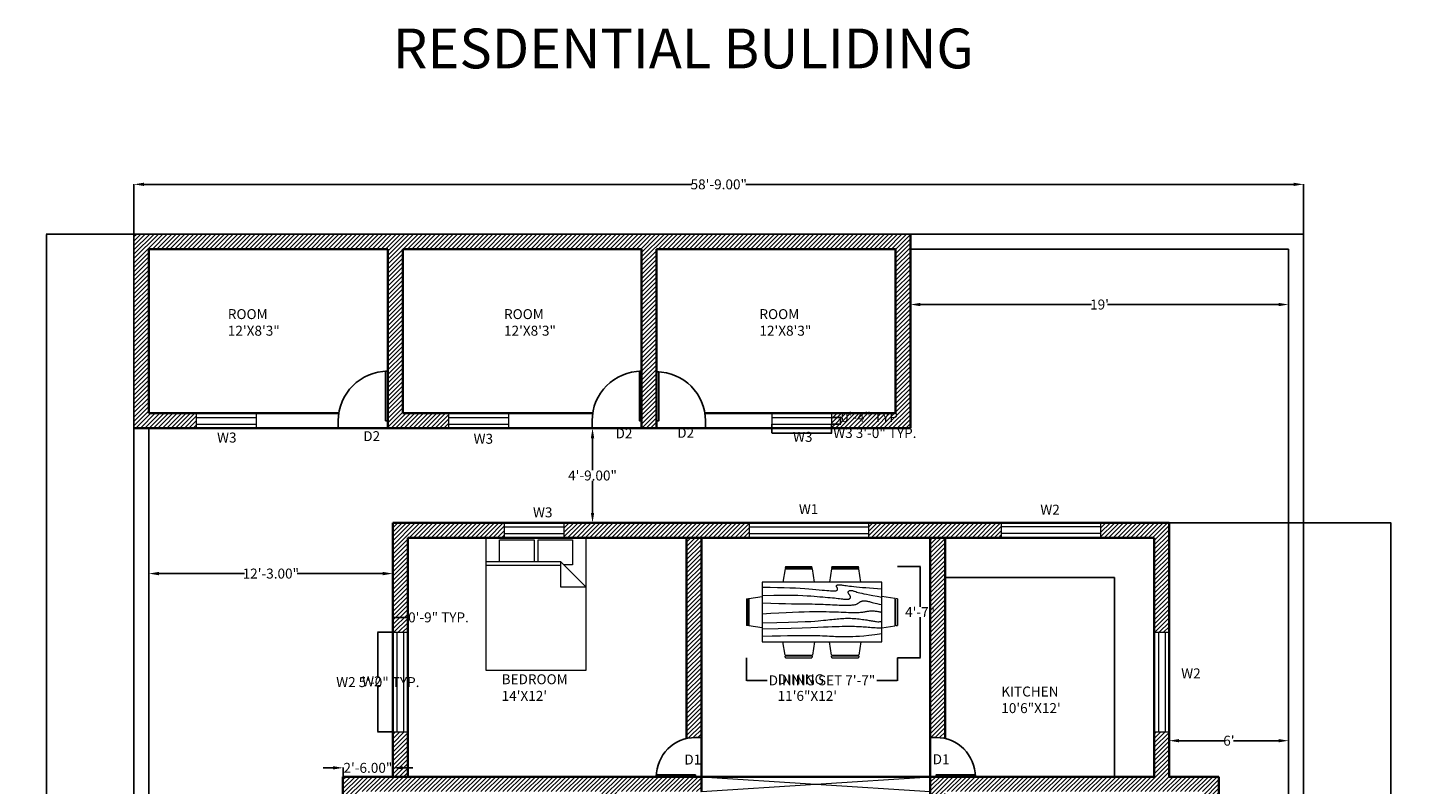
# Model space of a CAD drawing. Units: inches. Extents: x -57 to 1512, y -896 to 149.
# Tile 3 of 6: x -57 to 783, y -307 to 149. Entities that reach past the tile are written whole.
import ezdxf

# ---------------------------------------------------------------- set-up
doc = ezdxf.new("R2010")
doc.units = ezdxf.units.IN
doc.header["$MEASUREMENT"] = 0
doc.layers.get('Defpoints').update_dxf_attribs({"color": 9})
for name, color, linetype, lineweight in [('A-ANNO-DIMS', 2, 'Continuous', 18), ('A-ANNO-TEXT', 7, 'Continuous', 18), ('A-ANNO-TITL', 7, 'Continuous', 35), ('A-AREA-IDEN', 7, 'Continuous', 18), ('A-DOOR', 3, 'Continuous', 25), ('A-FLOR-CASE', 8, 'Continuous', 25), ('A-FURN', 8, 'Continuous', 18), ('A-GLAZ', 4, 'Continuous', 18), ('A-WALL', 7, 'Continuous', 35), ('A-WALL-OPEN', 7, 'Continuous', 18), ('A-WALL-PATT', 8, 'Continuous', 13), ('C-PROP', 7, 'Continuous', 25)]:
    doc.layers.add(name, color=color, linetype=linetype, lineweight=lineweight)
doc.styles.get("Standard").update_dxf_attribs({"font": 'arial.ttf'})
doc.dimstyles.get("Standard").update_dxf_attribs({"dimtxt": 6, "dimasz": 0.18, "dimexe": 0.18, "dimexo": 0.0625, "dimgap": 0.09, "dimtad": 0, "dimtih": 1, "dimtoh": 1, "dimzin": 0, "dimdsep": 46, "dimlunit": 3, "dimtxsty": 'Standard', "dimcen": 0.09, "dimadec": 0, "dimazin": 0, "dimtfac": 1, "dimtofl": 0, "dimtmove": 0, "dimatfit": 3, "dimfxl": 1, "dimtolj": 1, "dimtzin": 0, "dimarcsym": 0})

# ---------------------------------------------------------------- blocks, each defined once
blk = doc.blocks.new('*U2')
for p, q in [((0, 0), (0, -6)), ((40, 0), (40, -6))]:
    blk.add_line(p, q)
blk.add_lwpolyline([(0, 0), (0, 40), (1.75, 40), (1.75, 0)], close=True)
blk.add_arc((0, 0), 40, 0, 90)
blk = doc.blocks.new('Bed - Queen')
for p, q in [((0, -80.00003), (0, 0)), ((0, 0), (59.99999, 0)), ((59.99999, 0), (59.99999, -80.00003)), ((7.99999, -1.2), (28.79998, -1.2)), ((7.99999, -14.4), (7.99999, -1.2)), ((28.79998, -1.2), (28.79998, -14.4)), ((31.19999, -1.2), (51.99999, -1.2)), ((31.19999, -14.4), (31.19999, -1.2)), ((51.99999, -1.2), (51.99999, -16.4)), ((0, -14.4), (44.8, -14.4)), ((59.99999, -29.6), (44.8, -14.4)), ((44.8, -14.4), (44.8, -29.6)), ((51.99999, -16.4), (46.79936, -16.4)), ((44.8, -16.8), (0, -16.8)), ((44.8, -29.6), (59.99999, -29.6)), ((59.99999, -80.00003), (0, -80.00003))]:
    blk.add_line(p, q)
blk = doc.blocks.new('*D7')
at = {"layer": 'A-ANNO-DIMS', "color": 0, "lineweight": -2, "transparency": 16777216}
for p, q in [((283.51, -92.26), (283.88, -92.26)), ((283.7, -98.26), (283.7, -117.61)), ((283.7, -143.26), (283.7, -123.91)), ((283.51, -149.26), (283.88, -149.26))]:
    blk.add_line(p, q, dxfattribs=at)
at = {"layer": 'A-ANNO-DIMS', "color": 0, "transparency": 16777216}
for points in [[(282.7, -98.26), (284.7, -98.26), (283.7, -92.26)], [(282.7, -143.26), (284.7, -143.26), (283.7, -149.26)]]:
    blk.add_solid(points, dxfattribs=at)
at = {"layer": 'Defpoints', "color": 0, "transparency": 16777216}
for p in [(283.45, -92.26), (283.45, -149.26), (283.7, -149.26)]:
    blk.add_point(p, dxfattribs=at)
at = {"layer": 'A-ANNO-DIMS', "color": 0, "transparency": 16777216, "insert": (283.7, -120.76), "char_height": 6, "attachment_point": 5}
blk.add_mtext('\\A1;4\'-9.00"', dxfattribs=at)
blk = doc.blocks.new('*D8')
at = {"layer": 'A-ANNO-DIMS', "color": 0, "lineweight": -2, "transparency": 16777216}
for p, q in [((475.3, 15.68), (475.3, -17.9)), ((703.3, 15.68), (703.3, -17.9)), ((481.3, -17.72), (584.4, -17.72)), ((697.3, -17.72), (594.19, -17.72))]:
    blk.add_line(p, q, dxfattribs=at)
at = {"layer": 'A-ANNO-DIMS', "color": 0, "transparency": 16777216}
for points in [[(481.3, -16.72), (481.3, -18.72), (475.3, -17.72)], [(697.3, -16.72), (697.3, -18.72), (703.3, -17.72)]]:
    blk.add_solid(points, dxfattribs=at)
at = {"layer": 'Defpoints', "color": 0, "transparency": 16777216}
for p in [(475.3, 15.74), (703.3, 15.74), (703.3, -17.72)]:
    blk.add_point(p, dxfattribs=at)
at = {"layer": 'A-ANNO-DIMS', "color": 0, "transparency": 16777216, "insert": (589.3, -17.72), "char_height": 6, "attachment_point": 5}
blk.add_mtext("\\A1;19'", dxfattribs=at)
blk = doc.blocks.new('*D9')
at = {"layer": 'A-ANNO-DIMS', "color": 0, "lineweight": -2, "transparency": 16777216}
for p, q in [((661.3, -302.32), (661.3, -335.07)), ((703.3, -302.32), (703.3, -335.07)), ((667.3, -334.89), (668.41, -334.89)), ((697.3, -334.89), (696.18, -334.89))]:
    blk.add_line(p, q, dxfattribs=at)
at = {"layer": 'A-ANNO-DIMS', "color": 0, "transparency": 16777216}
for points in [[(667.3, -333.89), (667.3, -335.89), (661.3, -334.89)], [(697.3, -333.89), (697.3, -335.89), (703.3, -334.89)]]:
    blk.add_solid(points, dxfattribs=at)
at = {"layer": 'Defpoints', "color": 0, "transparency": 16777216}
for p in [(661.3, -302.26), (703.3, -302.26), (703.3, -334.89)]:
    blk.add_point(p, dxfattribs=at)
at = {"layer": 'A-ANNO-DIMS', "color": 0, "transparency": 16777216, "insert": (682.3, -334.89), "char_height": 6, "attachment_point": 5}
blk.add_mtext('\\A1;3\'-6.00"', dxfattribs=at)
blk = doc.blocks.new('*D18')
at = {"layer": 'A-ANNO-DIMS', "color": 0, "lineweight": -2, "transparency": 16777216}
for p, q in [((16.3, -149.32), (16.3, -180.04)), ((163.3, -149.32), (163.3, -180.04)), ((22.3, -179.86), (73.86, -179.86)), ((157.3, -179.86), (105.74, -179.86))]:
    blk.add_line(p, q, dxfattribs=at)
at = {"layer": 'A-ANNO-DIMS', "color": 0, "transparency": 16777216}
for points in [[(22.3, -178.86), (22.3, -180.86), (16.3, -179.86)], [(157.3, -178.86), (157.3, -180.86), (163.3, -179.86)]]:
    blk.add_solid(points, dxfattribs=at)
at = {"layer": 'Defpoints', "color": 0, "transparency": 16777216}
for p in [(16.3, -149.26), (163.3, -149.26), (16.3, -179.86)]:
    blk.add_point(p, dxfattribs=at)
at = {"layer": 'A-ANNO-DIMS', "color": 0, "transparency": 16777216, "insert": (89.8, -179.86), "char_height": 6, "attachment_point": 5}
blk.add_mtext('\\A1;12\'-3.00"', dxfattribs=at)
blk = doc.blocks.new('*D19')
at = {"layer": 'A-ANNO-DIMS', "color": 0, "lineweight": -2, "transparency": 16777216}
for p, q in [((16.3, -302.32), (16.3, -350.65)), ((133.3, -302.32), (133.3, -350.65)), ((22.3, -350.47), (60.91, -350.47)), ((127.3, -350.47), (88.69, -350.47))]:
    blk.add_line(p, q, dxfattribs=at)
at = {"layer": 'A-ANNO-DIMS', "color": 0, "transparency": 16777216}
for points in [[(22.3, -349.47), (22.3, -351.47), (16.3, -350.47)], [(127.3, -349.47), (127.3, -351.47), (133.3, -350.47)]]:
    blk.add_solid(points, dxfattribs=at)
at = {"layer": 'Defpoints', "color": 0, "transparency": 16777216}
for p in [(16.3, -302.26), (133.3, -302.26), (16.3, -350.47)]:
    blk.add_point(p, dxfattribs=at)
at = {"layer": 'A-ANNO-DIMS', "color": 0, "transparency": 16777216, "insert": (74.8, -350.47), "char_height": 6, "attachment_point": 5}
blk.add_mtext('\\A1;9\'-9.00"', dxfattribs=at)
blk = doc.blocks.new('*D20')
at = {"layer": 'A-ANNO-DIMS', "color": 0, "lineweight": -2, "transparency": 16777216}
for p, q in [((7.3, 24.8), (7.3, 54.88)), ((13.3, 54.7), (343.57, 54.7)), ((706.3, 54.7), (376.02, 54.7)), ((712.3, 24.8), (712.3, 54.88))]:
    blk.add_line(p, q, dxfattribs=at)
at = {"layer": 'A-ANNO-DIMS', "color": 0, "transparency": 16777216}
for points in [[(13.3, 55.7), (13.3, 53.7), (7.3, 54.7)], [(706.3, 55.7), (706.3, 53.7), (712.3, 54.7)]]:
    blk.add_solid(points, dxfattribs=at)
at = {"layer": 'Defpoints', "color": 0, "transparency": 16777216}
for p in [(7.3, 54.7), (7.3, 24.74), (712.3, 24.74)]:
    blk.add_point(p, dxfattribs=at)
at = {"layer": 'A-ANNO-DIMS', "color": 0, "transparency": 16777216, "insert": (359.8, 54.7), "char_height": 6, "attachment_point": 5}
blk.add_mtext('\\A1;58\'-9.00"', dxfattribs=at)
blk = doc.blocks.new('*D25')
at = {"layer": 'A-ANNO-DIMS', "color": 0, "lineweight": -2, "transparency": 16777216}
for p, q in [((631.3, -302.2), (631.3, -280.39)), ((637.3, -280.57), (664.43, -280.57)), ((697.3, -280.57), (670.16, -280.57)), ((703.3, -302.2), (703.3, -280.39))]:
    blk.add_line(p, q, dxfattribs=at)
at = {"layer": 'A-ANNO-DIMS', "color": 0, "transparency": 16777216}
for points in [[(637.3, -279.57), (637.3, -281.57), (631.3, -280.57)], [(697.3, -279.57), (697.3, -281.57), (703.3, -280.57)]]:
    blk.add_solid(points, dxfattribs=at)
at = {"layer": 'Defpoints', "color": 0, "transparency": 16777216}
for p in [(703.3, -280.57), (631.3, -302.26), (703.3, -302.26)]:
    blk.add_point(p, dxfattribs=at)
at = {"layer": 'A-ANNO-DIMS', "color": 0, "transparency": 16777216, "insert": (667.3, -280.57), "char_height": 6, "attachment_point": 5}
blk.add_mtext("\\A1;6'", dxfattribs=at)
blk = doc.blocks.new('*D26')
at = {"layer": 'A-ANNO-DIMS', "color": 0, "lineweight": -2, "transparency": 16777216}
for p, q in [((127.3, -296.93), (121.3, -296.93)), ((133.3, -302.2), (133.3, -296.75)), ((163.3, -302.2), (163.3, -296.75)), ((169.3, -296.93), (175.3, -296.93))]:
    blk.add_line(p, q, dxfattribs=at)
at = {"layer": 'A-ANNO-DIMS', "color": 0, "transparency": 16777216}
for points in [[(127.3, -295.93), (127.3, -297.93), (133.3, -296.93)], [(169.3, -295.93), (169.3, -297.93), (163.3, -296.93)]]:
    blk.add_solid(points, dxfattribs=at)
at = {"layer": 'Defpoints', "color": 0, "transparency": 16777216}
for p in [(163.3, -296.93), (133.3, -302.26), (163.3, -302.26)]:
    blk.add_point(p, dxfattribs=at)
at = {"layer": 'A-ANNO-DIMS', "color": 0, "transparency": 16777216, "insert": (148.3, -296.93), "char_height": 6, "attachment_point": 5}
blk.add_mtext('\\A1;2\'-6.00"', dxfattribs=at)
blk = doc.blocks.new('Dining Set - 36 x 72 in.')
for p, q in [((-22.2343, 26.00059), (-23.4847, 17.99762)), ((-22.2304, 26), (-5.7608, 26)), ((-22, 27.5), (-22.1562, 26.50042)), ((-5.8416, 26.5), (-22.1534, 26.5)), ((-22, 27.5), (-6, 27.5)), ((-5.8437, 26.49966), (-6, 27.5)), ((-4.5152, 17.99762), (-5.7655, 25.99926)), ((5.7657, 26.00059), (4.5153, 17.99762)), ((5.7696, 26), (22.2392, 26)), ((6, 27.5), (5.8438, 26.50042)), ((22.1584, 26.5), (5.8466, 26.5)), ((6, 27.5), (22, 27.5)), ((22.1563, 26.49966), (22, 27.5)), ((23.4848, 17.99762), (22.2345, 25.99926)), ((36, 18), (-36, 18)), ((-36, 18), (-36, -18)), ((36, -18), (36, 18)), ((-44.0006, 8.23428), (-35.9976, 9.48474)), ((44.0006, 8.23428), (35.9976, 9.48474)), ((-45.5, 8), (-44.5004, 8.15617)), ((-45.5, 8), (-45.5, -8)), ((-44.5, -8.15843), (-44.5, 8.15338)), ((-44, 8.23041), (-44, -8.23915)), ((44, 8.23041), (44, -8.23915)), ((44.5, -8.15843), (44.5, 8.15338)), ((45.5, 8), (44.5005, 8.15617)), ((45.5, 8), (45.5, -8)), ((-44.4997, -8.15631), (-45.5, -8)), ((-35.9976, -9.48476), (-43.9993, -8.2345)), ((35.9976, -9.48476), (43.9993, -8.2345)), ((44.4997, -8.15631), (45.5, -8)), ((-36, -18), (36, -18)), ((-22.2343, -26.0006), (-23.4847, -17.99762)), ((-4.5152, -17.99762), (-5.7655, -25.99928)), ((5.7657, -26.0006), (4.5153, -17.99762)), ((23.4848, -17.99762), (22.2345, -25.99928)), ((-22.2304, -26), (-5.7608, -26)), ((-22, -27.5), (-22.1562, -26.50044)), ((-5.8416, -26.5), (-22.1534, -26.5)), ((-22, -27.5), (-6, -27.5)), ((-5.8437, -26.49967), (-6, -27.5)), ((5.7696, -26), (22.2392, -26)), ((6, -27.5), (5.8438, -26.50044)), ((22.1584, -26.5), (5.8466, -26.5)), ((6, -27.5), (22, -27.5)), ((22.1563, -26.49967), (22, -27.5))]:
    blk.add_line(p, q)
for points in [[(-36, 15), (-31.1772, 14.97754), (-26.8079, 14.91406), (-22.8538, 14.81543), (-19.276, 14.6875), (-16.0362, 14.53613), (-13.0957, 14.36718), (-10.4159, 14.18652), (-7.9583, 14), (-5.6904, 13.81315), (-3.6035, 13.63021), (-1.6954, 13.45508), (0.0365, 13.29166), (1.5945, 13.14388), (2.9811, 13.01562), (4.1988, 12.9108), (5.25, 12.83333), (6.1393, 12.78613), (6.8802, 12.76823), (7.4883, 12.77767), (7.9792, 12.8125), (8.3685, 12.87077), (8.6719, 12.95052), (8.9049, 13.0498), (9.0833, 13.16666), (9.2205, 13.29899), (9.3216, 13.44401), (9.3895, 13.59879), (9.4271, 13.76041), (9.4373, 13.92594), (9.4232, 14.09245), (9.3875, 14.257), (9.3333, 14.41666), (9.2638, 14.56917), (9.1836, 14.71484), (9.0975, 14.85465), (9.0104, 14.98958), (8.9272, 15.1206), (8.8529, 15.2487), (8.7922, 15.37483), (8.75, 15.5), (8.7305, 15.62467), (8.7344, 15.74739), (8.7617, 15.86621), (8.8125, 15.97916), (8.8867, 16.08431), (8.9844, 16.17968), (9.1055, 16.26334), (9.25, 16.33333), (9.4189, 16.38802), (9.6172, 16.42708), (9.8506, 16.45052), (10.125, 16.45833), (10.4463, 16.45052), (10.8203, 16.42708), (11.2529, 16.38802), (11.75, 16.33333), (12.3184, 16.26318), (12.9694, 16.17838), (13.7151, 16.07991), (14.5677, 15.96875), (15.5395, 15.84586), (16.6426, 15.71224), (17.8893, 15.56884), (19.2917, 15.41666), (20.859, 15.25667), (22.5879, 15.08984), (24.4721, 14.91715), (26.5052, 14.73958), (28.6809, 14.5581), (30.9929, 14.3737), (33.4347, 14.18733), (36, 14)], [(-36, 10), (-28.9766, 10.14274), (-23.1725, 10.20442), (-18.4241, 10.19775), (-14.5677, 10.13541), (-11.4399, 10.03011), (-8.877, 9.89453), (-6.7154, 9.74137), (-4.7917, 9.58333), (-2.9698, 9.43082), (-1.2246, 9.28515), (0.4415, 9.14534), (2.026, 9.01041), (3.5266, 8.87939), (4.9408, 8.7513), (6.266, 8.62516), (7.5, 8.5), (8.6411, 8.37549), (9.6914, 8.2539), (10.6538, 8.13818), (11.5312, 8.03125), (12.3267, 7.93603), (13.043, 7.85547), (13.6831, 7.79248), (14.25, 7.75), (14.7471, 7.7303), (15.1797, 7.73307), (15.5537, 7.75732), (15.875, 7.80208), (16.1494, 7.86637), (16.3828, 7.94922), (16.5811, 8.04964), (16.75, 8.16666), (16.8944, 8.29915), (17.0143, 8.44531), (17.1089, 8.60319), (17.1771, 8.77083), (17.218, 8.94629), (17.2305, 9.1276), (17.2137, 9.31282), (17.1667, 9.5), (17.0895, 9.6875), (16.987, 9.875), (16.8649, 10.0625), (16.7292, 10.25), (16.5856, 10.4375), (16.4401, 10.625), (16.2985, 10.8125), (16.1667, 11), (16.05, 11.18733), (15.9518, 11.3737), (15.8752, 11.5581), (15.8229, 11.73958), (15.798, 11.91715), (15.8034, 12.08984), (15.842, 12.25667), (15.9167, 12.41666), (16.0295, 12.56836), (16.1784, 12.70833), (16.3605, 12.83268), (16.5729, 12.9375), (16.8127, 13.01888), (17.0768, 13.07291), (17.3625, 13.0957), (17.6667, 13.08333), (17.9894, 13.03312), (18.3418, 12.94726), (18.7382, 12.82918), (19.1927, 12.68229), (19.7195, 12.51001), (20.3327, 12.31575), (21.0465, 12.10294), (21.875, 11.875), (22.8357, 11.63354), (23.959, 11.37304), (25.2786, 11.08618), (26.8282, 10.76562), (28.6414, 10.40405), (30.752, 9.99414), (33.1936, 9.52856), (36, 9)], [(-36, 5.5), (-30.7157, 5.3348), (-26.069, 5.20963), (-21.9946, 5.11767), (-18.4271, 5.05208), (-15.3009, 5.00602), (-12.5508, 4.97265), (-10.1112, 4.94515), (-7.9167, 4.91666), (-5.909, 4.88167), (-4.0586, 4.83984), (-2.3429, 4.79215), (-0.7396, 4.73958), (0.7739, 4.6831), (2.22, 4.6237), (3.6213, 4.56233), (5, 4.5), (6.373, 4.43782), (7.7344, 4.3776), (9.0723, 4.32129), (10.375, 4.27083), (11.6309, 4.22819), (12.8281, 4.19531), (13.9551, 4.17415), (15, 4.16666), (15.954, 4.17448), (16.819, 4.19791), (17.6001, 4.23698), (18.3021, 4.29166), (18.9299, 4.36198), (19.4883, 4.44791), (19.9823, 4.54948), (20.4167, 4.66666), (20.7969, 4.79899), (21.1302, 4.94401), (21.4245, 5.09879), (21.6875, 5.26041), (21.9271, 5.42594), (22.1511, 5.59245), (22.3672, 5.757), (22.5834, 5.91666), (22.8065, 6.06868), (23.0404, 6.21093), (23.2879, 6.34147), (23.5521, 6.45833), (23.8358, 6.55957), (24.142, 6.64323), (24.4735, 6.70735), (24.8334, 6.75), (25.2235, 6.76969), (25.642, 6.76692), (26.0858, 6.74267), (26.5521, 6.69791), (27.0379, 6.63362), (27.5404, 6.55078), (28.0565, 6.45036), (28.5834, 6.33333), (29.1242, 6.19987), (29.7071, 6.04687), (30.3661, 5.87044), (31.1354, 5.66666), (32.0493, 5.43164), (33.142, 5.16146), (34.4475, 4.85221), (36, 4.5)], [(-36, -1), (-30.7915, -0.6591), (-26.0195, -0.38216), (-21.6519, -0.16284), (-17.6563, 0.00521), (-14.0005, 0.12833), (-10.6523, 0.21289), (-7.5796, 0.26522), (-4.75, 0.29166), (-2.134, 0.29793), (0.2878, 0.28711), (2.5317, 0.26163), (4.6146, 0.22396), (6.5529, 0.17651), (8.3633, 0.12174), (10.0623, 0.06209), (11.6667, 0), (13.1899, -0.06201), (14.6341, -0.1211), (15.9982, -0.17432), (17.2813, -0.21875), (18.4823, -0.25147), (19.6003, -0.26953), (20.6343, -0.27002), (21.5834, -0.25), (22.4481, -0.20768), (23.2357, -0.14584), (23.9549, -0.06836), (24.6146, 0.02083), (25.2235, 0.11784), (25.7904, 0.21875), (26.3241, 0.31966), (26.8334, 0.41666), (27.3265, 0.50618), (27.8099, 0.58593), (28.2894, 0.65397), (28.7709, 0.70833), (29.2601, 0.74707), (29.763, 0.76823), (30.2855, 0.76985), (30.8334, 0.75), (31.4088, 0.70784), (31.9994, 0.64713), (32.589, 0.57275), (33.1615, 0.48958), (33.7008, 0.4025), (34.1908, 0.3164), (34.6153, 0.23616), (34.9584, 0.16666), (35.2099, 0.11165), (35.3848, 0.07031), (35.504, 0.04069), (35.5886, 0.02083), (35.6594, 0.00879), (35.7377, 0.0026), (35.8442, 0.00032), (36, 0)], [(-36, -6.5), (-27.1843, -6.31267), (-20.084, -6.1263), (-14.469, -5.9419), (-10.1094, -5.76042), (-6.7752, -5.58285), (-4.2363, -5.41016), (-2.2629, -5.24333), (-0.625, -5.08334), (0.8708, -4.93099), (2.2715, -4.78646), (3.5872, -4.64974), (4.8281, -4.52084), (6.0046, -4.39974), (7.127, -4.28646), (8.2053, -4.18099), (9.25, -4.08334), (10.2705, -3.99382), (11.2734, -3.91407), (12.2647, -3.84603), (13.25, -3.79167), (14.2354, -3.75293), (15.2266, -3.73177), (16.2295, -3.73015), (17.25, -3.75), (18.2912, -3.79248), (19.3451, -3.85547), (20.4009, -3.93604), (21.4479, -4.03125), (22.4754, -4.13819), (23.4727, -4.25391), (24.4289, -4.37549), (25.3334, -4.5), (26.1785, -4.62492), (26.9694, -4.74935), (27.7145, -4.87281), (28.4219, -4.99479), (29.1, -5.11483), (29.7572, -5.23242), (30.4016, -5.34709), (31.0417, -5.45834), (31.6837, -5.56437), (32.3262, -5.65821), (32.9658, -5.73153), (33.599, -5.77604), (34.2224, -5.78345), (34.8327, -5.74545), (35.4264, -5.65373), (36, -5.5)], [(-36, -10), (-26.4022, -9.81299), (-18.4675, -9.62891), (-11.9839, -9.45069), (-6.7396, -9.28125), (-2.5226, -9.12354), (0.8789, -8.98047), (3.6769, -8.85498), (6.0833, -8.75), (8.2767, -8.66765), (10.3021, -8.60677), (12.1712, -8.56543), (13.8958, -8.54167), (15.4876, -8.53353), (16.9583, -8.53907), (18.3197, -8.55632), (19.5834, -8.58334), (20.7616, -8.61841), (21.8685, -8.66081), (22.9188, -8.71004), (23.9271, -8.76563), (24.9081, -8.82707), (25.8763, -8.89388), (26.8465, -8.96558), (27.8334, -9.04167), (28.8474, -9.12118), (29.8828, -9.20117), (30.93, -9.27824), (31.9792, -9.34896), (33.0205, -9.40991), (34.0443, -9.45768), (35.0407, -9.48885), (36, -9.5)], [(-36, -14.5), (-30.0881, -14.33513), (-25.0332, -14.21224), (-20.7312, -14.12647), (-17.0781, -14.07292), (-13.97, -14.04671), (-11.3027, -14.04297), (-8.9724, -14.05681), (-6.875, -14.08334), (-4.9224, -14.11833), (-3.0905, -14.16016), (-1.3709, -14.20785), (0.2448, -14.26042), (1.7647, -14.3169), (3.1973, -14.3763), (4.5507, -14.43767), (5.8333, -14.5), (7.0554, -14.5621), (8.235, -14.62175), (9.3922, -14.67652), (10.5469, -14.72396), (11.7192, -14.76164), (12.929, -14.78711), (14.1965, -14.79794), (15.5417, -14.79167), (16.9933, -14.76424), (18.6152, -14.70508), (20.4804, -14.60197), (22.6615, -14.44271), (25.2312, -14.21509), (28.2624, -13.9069), (31.8277, -13.50594), (36, -13)]]:
    blk.add_lwpolyline(points)
blk = doc.blocks.new('GLAZ-SASH-36IN')
for p, q in [((0, 4), (36, 4)), ((0, 0), (36, 0))]:
    blk.add_line(p, q)
blk = doc.blocks.new('WIN-60IN')
for p, q in [((0, 60), (9, 60)), ((2.5, 60), (2.5, 0)), ((6.5, 60), (6.5, 0)), ((0, 0), (9, 0))]:
    blk.add_line(p, q)
blk = doc.blocks.new('WIN-72IN')
for p, q in [((0, 0), (0, 9)), ((72, 0), (72, 9)), ((0, 6.5), (72, 6.5)), ((0, 2.5), (72, 2.5))]:
    blk.add_line(p, q)
blk = doc.blocks.new('*D93')
at = {"layer": 'A-ANNO-DIMS', "color": 0, "lineweight": -2, "transparency": 16777216}
for p, q in [((391.77, -89.82), (391.77, -95.34)), ((427.77, -89.82), (427.77, -95.34)), ((391.95, -95.16), (427.59, -95.16)), ((427.77, -95.16), (427.95, -95.16))]:
    blk.add_line(p, q, dxfattribs=at)
at = {"layer": 'A-ANNO-DIMS', "color": 0, "transparency": 16777216}
for points in [[(391.95, -95.13), (391.95, -95.19), (391.77, -95.16)], [(427.59, -95.13), (427.59, -95.19), (427.77, -95.16)]]:
    blk.add_solid(points, dxfattribs=at)
at = {"layer": 'Defpoints', "color": 0, "transparency": 16777216}
for p in [(391.77, -89.76), (427.77, -89.76), (427.77, -95.16)]:
    blk.add_point(p, dxfattribs=at)
at = {"layer": 'A-ANNO-DIMS', "color": 0, "transparency": 16777216, "insert": (453.9, -95.16), "char_height": 6, "attachment_point": 5}
blk.add_mtext('\\A1;W3 3\'-0" TYP.', dxfattribs=at)
blk = doc.blocks.new('*D94')
at = {"layer": 'A-ANNO-DIMS', "color": 0, "lineweight": -2, "transparency": 16777216}
for p, q in [((427.83, -85.76), (433.35, -85.76)), ((427.83, -89.76), (433.35, -89.76)), ((433.17, -85.76), (433.17, -85.58)), ((433.17, -85.58), (433.35, -85.58)), ((433.17, -89.58), (433.17, -85.94))]:
    blk.add_line(p, q, dxfattribs=at)
at = {"layer": 'A-ANNO-DIMS', "color": 0, "transparency": 16777216}
for points in [[(433.14, -85.94), (433.2, -85.94), (433.17, -85.76)], [(433.14, -89.58), (433.2, -89.58), (433.17, -89.76)]]:
    blk.add_solid(points, dxfattribs=at)
at = {"layer": 'Defpoints', "color": 0, "transparency": 16777216}
for p in [(427.77, -85.76), (427.77, -89.76), (433.17, -85.76)]:
    blk.add_point(p, dxfattribs=at)
at = {"layer": 'A-ANNO-DIMS', "color": 0, "transparency": 16777216, "insert": (451.73, -85.58), "char_height": 6, "attachment_point": 5}
blk.add_mtext('\\A1;0\'-4" TYP.', dxfattribs=at)
blk = doc.blocks.new('*D99')
at = {"layer": 'A-ANNO-DIMS', "color": 0, "lineweight": -2, "transparency": 16777216}
for p, q in [((163.23, -215.26), (154.12, -215.26)), ((154.3, -215.44), (154.3, -242.11)), ((154.3, -275.08), (154.3, -248.41)), ((163.23, -275.26), (154.12, -275.26))]:
    blk.add_line(p, q, dxfattribs=at)
at = {"layer": 'A-ANNO-DIMS', "color": 0, "transparency": 16777216}
for points in [[(154.27, -215.44), (154.33, -215.44), (154.3, -215.26)], [(154.27, -275.08), (154.33, -275.08), (154.3, -275.26)]]:
    blk.add_solid(points, dxfattribs=at)
at = {"layer": 'Defpoints', "color": 0, "transparency": 16777216}
for p in [(154.3, -215.26), (163.3, -215.26), (163.3, -275.26)]:
    blk.add_point(p, dxfattribs=at)
at = {"layer": 'A-ANNO-DIMS', "color": 0, "transparency": 16777216, "insert": (154.3, -245.26), "char_height": 6, "attachment_point": 5}
blk.add_mtext('\\A1;W2 5\'-0" TYP.', dxfattribs=at)
blk = doc.blocks.new('*D100')
at = {"layer": 'A-ANNO-DIMS', "color": 0, "lineweight": -2, "transparency": 16777216}
for p, q in [((163.3, -215.2), (163.3, -206.08)), ((163.48, -206.26), (172.12, -206.26)), ((172.3, -215.2), (172.3, -206.08)), ((172.3, -206.26), (172.48, -206.26))]:
    blk.add_line(p, q, dxfattribs=at)
at = {"layer": 'A-ANNO-DIMS', "color": 0, "transparency": 16777216}
for points in [[(163.48, -206.23), (163.48, -206.29), (163.3, -206.26)], [(172.12, -206.23), (172.12, -206.29), (172.3, -206.26)]]:
    blk.add_solid(points, dxfattribs=at)
at = {"layer": 'Defpoints', "color": 0, "transparency": 16777216}
for p in [(172.3, -206.26), (163.3, -215.26), (172.3, -215.26)]:
    blk.add_point(p, dxfattribs=at)
at = {"layer": 'A-ANNO-DIMS', "color": 0, "transparency": 16777216, "insert": (190.85, -206.26), "char_height": 6, "attachment_point": 5}
blk.add_mtext('\\A1;0\'-9" TYP.', dxfattribs=at)
blk = doc.blocks.new('*D101')
at = {"layer": 'A-ANNO-DIMS', "color": 0, "lineweight": -2, "transparency": 16777216}
for p, q in [((376.5, -230.63), (376.5, -244.4)), ((467.5, -230.63), (467.5, -244.4)), ((376.68, -244.22), (388.93, -244.22)), ((467.32, -244.22), (455.06, -244.22))]:
    blk.add_line(p, q, dxfattribs=at)
at = {"layer": 'A-ANNO-DIMS', "color": 0, "transparency": 16777216}
for points in [[(376.68, -244.19), (376.68, -244.25), (376.5, -244.22)], [(467.32, -244.19), (467.32, -244.25), (467.5, -244.22)]]:
    blk.add_solid(points, dxfattribs=at)
at = {"layer": 'Defpoints', "color": 0, "transparency": 16777216}
for p in [(376.5, -230.57), (467.5, -230.57), (467.5, -244.22)]:
    blk.add_point(p, dxfattribs=at)
at = {"layer": 'A-ANNO-DIMS', "color": 0, "transparency": 16777216, "insert": (422, -244.22), "char_height": 6, "attachment_point": 5}
blk.add_mtext('\\A1;DINING SET 7\'-7"', dxfattribs=at)
blk = doc.blocks.new('*D102')
at = {"layer": 'A-ANNO-DIMS', "color": 0, "lineweight": -2, "transparency": 16777216}
for p, q in [((467.56, -175.57), (481.33, -175.57)), ((481.15, -175.75), (481.15, -199.98)), ((481.15, -230.39), (481.15, -206.16)), ((467.56, -230.57), (481.33, -230.57))]:
    blk.add_line(p, q, dxfattribs=at)
at = {"layer": 'A-ANNO-DIMS', "color": 0, "transparency": 16777216}
for points in [[(481.12, -175.75), (481.18, -175.75), (481.15, -175.57)], [(481.12, -230.39), (481.18, -230.39), (481.15, -230.57)]]:
    blk.add_solid(points, dxfattribs=at)
at = {"layer": 'Defpoints', "color": 0, "transparency": 16777216}
for p in [(467.5, -175.57), (481.15, -175.57), (467.5, -230.57)]:
    blk.add_point(p, dxfattribs=at)
at = {"layer": 'A-ANNO-DIMS', "color": 0, "transparency": 16777216, "insert": (481.15, -203.07), "char_height": 6, "attachment_point": 5}
blk.add_mtext('\\A1;4\'-7"', dxfattribs=at)
blk = doc.blocks.new('*D103')
at = {"layer": 'A-ANNO-DIMS', "color": 0, "lineweight": -2, "transparency": 16777216}
for p, q in [((7.23, 24.74), (-45.53, 24.74)), ((-45.35, 24.56), (-45.35, -428.11)), ((-45.35, -887.08), (-45.35, -434.41)), ((7.23, -887.26), (-45.53, -887.26))]:
    blk.add_line(p, q, dxfattribs=at)
at = {"layer": 'A-ANNO-DIMS', "color": 0, "transparency": 16777216}
for points in [[(-45.38, 24.56), (-45.32, 24.56), (-45.35, 24.74)], [(-45.38, -887.08), (-45.32, -887.08), (-45.35, -887.26)]]:
    blk.add_solid(points, dxfattribs=at)
at = {"layer": 'Defpoints', "color": 0, "transparency": 16777216}
for p in [(-45.35, 24.74), (7.3, 24.74), (7.3, -887.26)]:
    blk.add_point(p, dxfattribs=at)
at = {"layer": 'A-ANNO-DIMS', "color": 0, "transparency": 16777216, "insert": (-45.35, -431.26), "char_height": 6, "attachment_point": 5}
blk.add_mtext('\\A1;76\'-0"', dxfattribs=at)
blk = doc.blocks.new('*D104')
at = {"layer": 'A-ANNO-DIMS', "color": 0, "lineweight": -2, "transparency": 16777216}
for p, q in [((631.36, -149.26), (765.13, -149.26)), ((764.95, -149.44), (764.95, -437.82)), ((764.95, -732.58), (764.95, -444.2)), ((661.36, -732.76), (765.13, -732.76))]:
    blk.add_line(p, q, dxfattribs=at)
at = {"layer": 'A-ANNO-DIMS', "color": 0, "transparency": 16777216}
for points in [[(764.92, -149.44), (764.98, -149.44), (764.95, -149.26)], [(764.92, -732.58), (764.98, -732.58), (764.95, -732.76)]]:
    blk.add_solid(points, dxfattribs=at)
at = {"layer": 'Defpoints', "color": 0, "transparency": 16777216}
for p in [(631.3, -149.26), (764.95, -149.26), (661.3, -732.76)]:
    blk.add_point(p, dxfattribs=at)
at = {"layer": 'A-ANNO-DIMS', "color": 0, "transparency": 16777216, "insert": (764.95, -441.01), "char_height": 6, "attachment_point": 5}
blk.add_mtext('\\A1;48\'-7 1/2"', dxfattribs=at)

msp = doc.modelspace()

# ---------------------------------------------------------------- hatches: boundary and pattern name
at = {"layer": 'A-WALL-PATT'}
h = msp.add_hatch(dxfattribs=at)
h.set_pattern_fill('ANSI31', color=256, scale=15)
h.paths.add_polyline_path([(322.296, 15.74), (466.296, 15.74), (466.296, -83.26), (427.769, -83.26), (427.769, -92.26), (475.296, -92.26), (475.296, 24.74), (7.296, 24.74), (7.296, -92.26), (44.859, -92.26), (44.859, -83.26), (16.296, -83.26), (16.296, 15.74), (160.296, 15.74), (160.296, -92.26), (196.971, -92.26), (196.971, -83.26), (169.296, -83.26), (169.296, 15.74), (313.296, 15.74), (313.296, -92.26), (322.296, -92.26), (322.296, -87.833), (322.296, -58.321)])
h = msp.add_hatch(dxfattribs=at)
h.set_pattern_fill('ANSI31', color=256, scale=15)
h.paths.add_polyline_path([(496.296, -570.76), (487.296, -570.76), (474.037, -570.76), (474.037, -579.76), (487.296, -579.76), (487.296, -732.76), (545.372, -732.76), (545.372, -723.76), (496.296, -723.76)])
h.paths.add_polyline_path([(661.296, -684.034), (652.296, -684.034), (652.296, -723.76), (617.372, -723.76), (617.372, -732.76), (661.296, -732.76)])
h.paths.add_polyline_path([(298.296, -570.76), (208.296, -570.76), (208.296, -575.26), (172.296, -575.26), (172.296, -534.76), (163.296, -534.76), (163.296, -604.062), (172.296, -604.062), (172.296, -579.76), (298.296, -579.76)])
h.paths.add_polyline_path([(172.296, -494.26), (163.296, -494.26), (163.296, -498.76), (172.296, -498.76)])
h.paths.add_polyline_path([(242.796, -494.26), (172.296, -494.26), (172.296, -498.76), (238.296, -498.76), (242.796, -498.76)])
h.paths.add_polyline_path([(242.796, -522.76), (238.296, -522.76), (238.296, -570.76), (242.796, -570.76)])
h.paths.add_polyline_path([(142.296, -405.989), (133.296, -405.989), (133.296, -458.26), (250.953, -458.26), (250.953, -452.508, -0.0212094), (251.091, -449.26), (142.296, -449.26)])
h.paths.add_polyline_path([(298.296, -311.26), (349.296, -311.26), (349.296, -302.26), (345.753, -302.26), (322.135, -302.26), (133.296, -302.26), (133.296, -345.989), (142.296, -345.989), (142.296, -311.26), (289.296, -311.26), (289.296, -458.26), (298.296, -458.26)])
h.paths.add_polyline_path([(172.296, -275.26), (163.296, -275.26), (163.296, -302.26), (172.296, -302.26)])
h.paths.add_polyline_path([(172.296, -158.26), (230.655, -158.26), (230.655, -149.26), (163.296, -149.26), (163.296, -215.26), (172.296, -215.26)])
h.paths.add_polyline_path([(378.235, -149.26), (266.655, -149.26), (266.655, -158.26), (378.235, -158.26)])
h.paths.add_polyline_path([(349.296, -158.26), (340.296, -158.26), (340.296, -279.28, -0.0583572), (345.753, -278.641), (349.296, -278.641)])
h.paths.add_polyline_path([(529.979, -149.26), (450.235, -149.26), (450.235, -158.26), (529.979, -158.26)])
h.paths.add_polyline_path([(496.296, -158.26), (487.296, -158.26), (487.296, -278.641), (490.839, -278.641, -0.0583572), (496.296, -279.28)])
h.paths.add_polyline_path([(631.296, -149.26), (589.979, -149.26), (589.979, -158.26), (622.296, -158.26), (622.296, -215.26), (631.296, -215.26)])
h.paths.add_polyline_path([(661.296, -302.26), (631.296, -302.26), (631.296, -275.26), (622.296, -275.26), (622.296, -302.26), (487.296, -302.26), (487.296, -458.26), (496.296, -458.26), (496.296, -453.783), (496.296, -423.936), (496.296, -311.26), (652.296, -311.26), (652.296, -340.453), (661.296, -340.453)])
h.paths.add_polyline_path([(349.296, -579.76), (359.066, -579.76), (359.066, -570.76), (340.296, -570.76), (340.296, -682.249, -0.0275619), (344.104, -682.039), (349.296, -682.039)])
h.paths.add_polyline_path([(172.296, -676.062), (163.296, -676.062), (163.296, -732.76), (200.083, -732.76), (200.083, -723.76), (172.296, -723.76)])
h.paths.add_polyline_path([(349.296, -716.654), (344.104, -716.654), (340.296, -716.654), (340.296, -723.76), (272.083, -723.76), (272.083, -732.76), (349.296, -732.76)])

# ---------------------------------------------------------------- linework, layer by layer
at = {"layer": 'A-FLOR-CASE'}
for p, q in [((496.296, -182.26), (598.296, -182.26)), ((598.296, -182.26), (598.296, -302.26))]:
    msp.add_line(p, q, dxfattribs=at)
at = {"layer": 'A-GLAZ'}
for p, q in [((44.859, -83.26), (44.859, -92.26)), ((80.859, -83.26), (80.859, -92.26)), ((196.971, -83.26), (196.971, -92.26)), ((232.971, -83.26), (232.971, -92.26)), ((391.769, -83.26), (391.769, -92.26)), ((427.769, -83.26), (427.769, -92.26)), ((230.655, -158.26), (230.655, -149.26)), ((266.655, -158.26), (266.655, -149.26)), ((622.296, -215.26), (631.296, -215.26)), ((624.796, -215.26), (624.796, -275.26)), ((628.796, -215.26), (628.796, -275.26)), ((628.796, -215.26), (628.796, -275.26)), ((622.296, -275.26), (631.296, -275.26))]:
    msp.add_line(p, q, dxfattribs=at)
at = {"layer": 'A-WALL'}
for p, q in [((475.296, 24.74), (475.296, -92.26)), ((16.296, 15.74), (160.296, 15.74)), ((16.296, 15.74), (16.296, -83.26)), ((160.296, 15.74), (160.296, -92.26)), ((169.296, 15.74), (169.296, -83.26)), ((169.296, 15.74), (313.296, 15.74)), ((313.296, 15.74), (313.296, -92.26)), ((322.296, 15.74), (322.296, -92.26)), ((322.296, 15.74), (466.296, 15.74)), ((466.296, 15.74), (466.296, -83.26)), ((16.296, -83.26), (130.793, -83.26)), ((169.296, -83.26), (283.795, -83.26)), ((351.451, -83.26), (466.296, -83.26)), ((7.296, -92.26), (475.296, -92.26)), ((163.296, -149.26), (631.296, -149.26)), ((163.296, -149.26), (163.296, -302.26)), ((631.296, -149.26), (631.296, -302.26)), ((172.296, -158.26), (622.296, -158.26)), ((172.296, -158.26), (172.296, -302.26)), ((340.296, -158.26), (340.296, -279.28)), ((349.296, -158.26), (349.296, -311.26)), ((487.296, -158.26), (487.296, -302.26)), ((496.296, -158.26), (496.296, -279.28)), ((622.296, -158.26), (622.296, -302.26)), ((133.296, -302.26), (133.296, -458.26)), ((133.296, -302.26), (622.296, -302.26)), ((487.296, -302.26), (487.296, -570.76)), ((631.296, -302.26), (661.296, -302.26)), ((661.296, -302.26), (661.296, -458.26))]:
    msp.add_line(p, q, dxfattribs=at)
at = {"layer": 'A-WALL-OPEN'}
for p, q in [((349.296, -302.26), (487.296, -311.26)), ((349.296, -311.26), (487.296, -302.26))]:
    msp.add_line(p, q, dxfattribs=at)
at = {"layer": 'C-PROP'}
for p, q in [((7.296, 24.74), (712.296, 24.74)), ((7.296, 24.74), (7.296, -887.26)), ((712.296, 24.74), (712.296, -887.26)), ((475.296, 15.74), (703.296, 15.74)), ((703.296, 15.74), (703.296, -302.26)), ((16.296, -92.26), (16.296, -158.26)), ((16.296, -158.26), (16.296, -302.26)), ((16.296, -302.26), (16.296, -458.26)), ((703.296, -302.26), (703.296, -458.26))]:
    msp.add_line(p, q, dxfattribs=at)

# ---------------------------------------------------------------- block references
at = {"layer": 'A-DOOR'}
for p, xscale, yscale, zscale in [((160.296, -87.782), -0.7461927941316632, 0.7461927941316632, 0.7461927941316632), ((313.296, -87.783), -0.7461532224003351, 0.7461532224003351, 0.7461532224003351), ((322.296, -87.833), 0.7377834374664785, 0.7377834374664785, 0.7377834374664785)]:
    msp.add_blockref('*U2', p, dxfattribs=dict(at, xscale=xscale, yscale=yscale, zscale=zscale))
at = {"layer": 'A-DOOR', "yscale": 0.5904621008807976, "zscale": 0.5904621008807976}
for p, xscale, rotation in [((345.753, -302.26), 0.5904621008807976, 90.00000000000003), ((490.839, -302.26), -0.5904621008807976, 270)]:
    msp.add_blockref('*U2', p, dxfattribs=dict(at, xscale=xscale, rotation=rotation))
at = {"layer": 'A-FURN'}
for name, p in [('Bed - Queen', (219.645, -158.26)), ('Dining Set - 36 x 72 in.', (421.998, -203.07))]:
    msp.add_blockref(name, p, dxfattribs=at)
at = {"layer": 'A-GLAZ'}
for name, p in [('GLAZ-SASH-36IN', (44.859, -89.76)), ('GLAZ-SASH-36IN', (196.971, -89.76)), ('GLAZ-SASH-36IN', (391.769, -89.76)), ('WIN-72IN', (378.235, -158.26)), ('GLAZ-SASH-36IN', (230.655, -155.76)), ('WIN-60IN', (163.296, -275.26))]:
    msp.add_blockref(name, p, dxfattribs=at)
at = {"layer": 'A-GLAZ', "rotation": 270.0000000000002}
msp.add_blockref('WIN-60IN', (529.978, -149.26), dxfattribs=at)

# ---------------------------------------------------------------- texts
at = {"layer": 'A-ANNO-TEXT', "char_height": 6, "attachment_point": 1}
for s, insert in [('D2', (297.584, -92.367)), ('D2', (334.767, -92.037)), ('W3', (57.387, -94.891)), ('D2', (145.495, -94.042)), ('W3', (212.021, -95.63)), ('W3', (404.552, -94.464)), ('W3', (247.818, -139.967)), ('W1', (408.114, -138.038)), ('W2', (553.639, -138.339)), ('W2', (144.845, -241.748)), ('W2', (638.55, -236.994)), ('D1', (339.064, -288.932)), ('D1', (488.741, -288.765))]:
    msp.add_mtext_dynamic_manual_height_columns(s, width=173.83392, gutter_width=1, heights=[0], dxfattribs=dict(at, insert=insert))
at = {"layer": 'A-ANNO-TITL', "insert": (163.381, 148.586), "char_height": 24, "attachment_point": 1}
msp.add_mtext_dynamic_manual_height_columns('RESDENTIAL BULIDING', width=777.91361, gutter_width=1, heights=[0], dxfattribs=at)
at = {"layer": 'A-AREA-IDEN', "char_height": 6, "attachment_point": 1}
for s, insert in [('ROOM\\P12\'X8\'3"', (63.876, -20.503)), ('ROOM\\P12\'X8\'3"', (230.355, -20.503)), ('ROOM\\P12\'X8\'3"', (384.308, -20.503)), ("BEDROOM\\P14'X12'", (228.917, -240.553)), ('DINING\\P11\'6"X12\'', (395.272, -240.553)), ('KITCHEN\\P10\'6"X12\'', (530.095, -247.944))]:
    msp.add_mtext_dynamic_manual_height_columns(s, width=160.11736, gutter_width=1, heights=[0], dxfattribs=dict(at, insert=insert))

# ---------------------------------------------------------------- dimensions: what is measured, and where the dimension line sits
at = {"layer": 'A-ANNO-DIMS'}
for base, p1, p2, picture, middle in [((7.296, 54.7), (712.296, 24.74), (7.296, 24.74), '*D20', (359.796, 54.7)), ((703.296, -17.722), (475.296, 15.74), (703.296, 15.74), '*D8', (589.296, -17.722)), ((16.296, -179.865), (163.296, -149.26), (16.296, -149.26), '*D18', (89.796, -179.865)), ((703.296, -280.567), (631.296, -302.26), (703.296, -302.26), '*D25', (667.296, -280.567)), ((163.296, -296.932), (133.296, -302.26), (163.296, -302.26), '*D26', (148.296, -296.932)), ((16.296, -350.472), (133.296, -302.26), (16.296, -302.26), '*D19', (74.796, -350.472)), ((703.296, -334.886), (661.296, -302.26), (703.296, -302.26), '*D9', (682.296, -334.886))]:
    dim = msp.add_linear_dim(base=base, p1=p1, p2=p2, dimstyle='Standard', override={"dimasz": 6, "dimclrd": 0, "dimclre": 0, "dimclrt": 0}, dxfattribs=at)
    dim.commit()
    dim.dimension.update_dxf_attribs({"geometry": picture, "text_midpoint": middle})
for base, p1, p2, override, picture, middle in [((-45.354, 24.74), (7.296, -887.26), (7.296, 24.74), {"dimdec": 1, "dimlfac": 1, "dimrnd": 0, "dimzin": 1, "dimdsep": 46, "dimlunit": 4, "dimfrac": 2}, '*D103', (-45.354, -431.26)), ((283.695, -149.26), (283.45, -92.26), (283.45, -149.26), {"dimasz": 6, "dimclrd": 0, "dimclre": 0, "dimclrt": 0}, '*D7', (283.695, -120.76)), ((764.946, -149.26), (661.296, -732.76), (631.296, -149.26), {"dimdec": 1, "dimlfac": 1, "dimrnd": 0, "dimzin": 1, "dimdsep": 46, "dimlunit": 4, "dimfrac": 2}, '*D104', (764.946, -441.01)), ((481.148, -175.57), (467.498, -230.57), (467.498, -175.57), {"dimdec": 1, "dimlfac": 1, "dimrnd": 0, "dimzin": 1, "dimdsep": 46, "dimlunit": 4, "dimfrac": 2}, '*D102', (481.148, -203.07))]:
    dim = msp.add_linear_dim(base=base, p1=p1, p2=p2, angle=90, dimstyle='Standard', override=override, dxfattribs=at)
    dim.commit()
    dim.dimension.update_dxf_attribs({"geometry": picture, "text_midpoint": middle})
for base, p1, p2, text, picture, middle in [((427.769, -95.16), (391.769, -89.76), (427.769, -89.76), 'W3 <> TYP.', '*D93', (453.899, -95.16)), ((172.296, -206.26), (163.296, -215.26), (172.296, -215.26), '<> TYP.', '*D100', (190.852, -206.26)), ((467.498, -244.22), (376.498, -230.57), (467.498, -230.57), 'DINING SET <>', '*D101', (421.998, -244.22))]:
    dim = msp.add_linear_dim(base=base, p1=p1, p2=p2, text=text, dimstyle='Standard', override={"dimdec": 1, "dimlfac": 1, "dimrnd": 0, "dimzin": 1, "dimdsep": 46, "dimlunit": 4, "dimfrac": 2}, dxfattribs=at)
    dim.commit()
    dim.dimension.update_dxf_attribs({"geometry": picture, "text_midpoint": middle})
for base, p1, p2, text, picture, middle in [((433.169, -85.76), (427.769, -89.76), (427.769, -85.76), '<> TYP.', '*D94', (451.726, -85.58)), ((154.296, -215.26), (163.296, -275.26), (163.296, -215.26), 'W2 <> TYP.', '*D99', (154.296, -245.26))]:
    dim = msp.add_linear_dim(base=base, p1=p1, p2=p2, angle=90, text=text, dimstyle='Standard', override={"dimdec": 1, "dimlfac": 1, "dimrnd": 0, "dimzin": 1, "dimdsep": 46, "dimlunit": 4, "dimfrac": 2}, dxfattribs=at)
    dim.commit()
    dim.dimension.update_dxf_attribs({"geometry": picture, "text_midpoint": middle})

doc.saveas('drawing.dxf')
